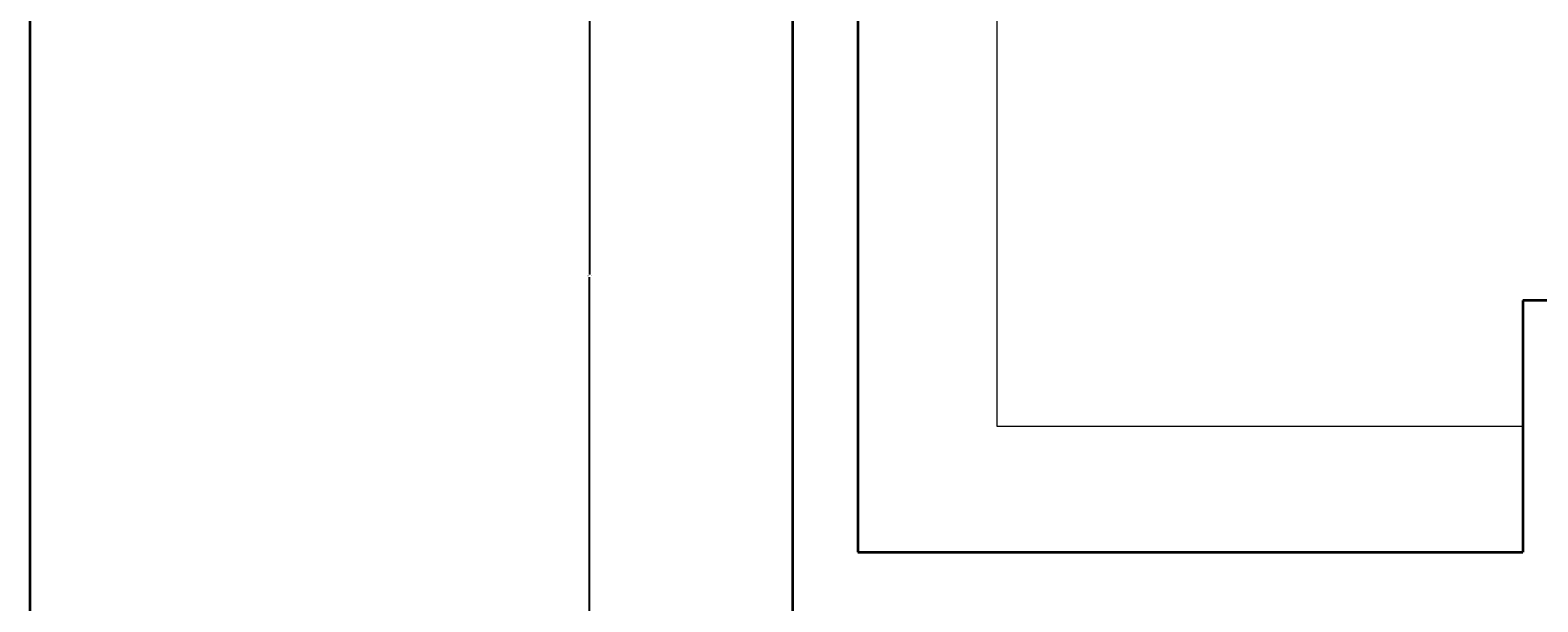
# Model space of a CAD drawing. Units: inches. Extents: x 1911 to 3278, y 2022 to 3108.
# Tile 6 of 13: x 1911 to 2120, y 2266 to 2345. Entities that reach past the tile are written whole.
import ezdxf

# ---------------------------------------------------------------- set-up
doc = ezdxf.new("R2010")
doc.units = ezdxf.units.IN
for name, color, linetype, lineweight in [('A-ANNO-DIMS', 2, 'Continuous', 18), ('A-ANNO-TTLB', 7, 'Continuous', 35), ('A-FLOR-CASE', 9, 'Continuous', 18), ('A-WALL', 7, 'Continuous', 35)]:
    doc.layers.add(name, color=color, linetype=linetype, lineweight=lineweight)
doc.styles.get("Standard").update_dxf_attribs({"font": 'arial.ttf'})
doc.dimstyles.get("Standard").update_dxf_attribs({"dimtxt": 0.18, "dimasz": 0.18, "dimexe": 0.18, "dimexo": 0.0625, "dimgap": 0.09, "dimtad": 0, "dimtih": 1, "dimtoh": 1, "dimdec": 4, "dimzin": 0, "dimdsep": 46, "dimtxsty": 'Standard', "dimcen": 0.09, "dimadec": 0, "dimazin": 0, "dimtfac": 1, "dimtdec": 4, "dimtofl": 0, "dimtmove": 0, "dimatfit": 3, "dimfxl": 1, "dimtolj": 1, "dimtzin": 0, "dimarcsym": 0})

# ---------------------------------------------------------------- blocks, each defined once
blk = doc.blocks.new('COUNTER-KITCHEN-L')
for p, q in [((19.27, 79.32), (0, 79.32)), ((19.27, 0), (19.27, 79.32)), ((92, 0), (19.27, 0))]:
    blk.add_line(p, q)
blk = doc.blocks.new('*D72')
at = {"layer": 'A-ANNO-DIMS', "color": 0, "lineweight": -2, "transparency": 16777216}
for p, q in [((2016.77, 2358.3), (1988.55, 2358.3)), ((1988.73, 2358.12), (1988.73, 2311.27)), ((1988.73, 2264.05), (1988.73, 2310.9)), ((2016.77, 2263.87), (1988.55, 2263.87))]:
    blk.add_line(p, q, dxfattribs=at)
at = {"layer": 'A-ANNO-DIMS', "color": 0, "transparency": 16777216}
for points in [[(1988.7, 2358.12), (1988.76, 2358.12), (1988.73, 2358.3)], [(1988.7, 2264.05), (1988.76, 2264.05), (1988.73, 2263.87)]]:
    blk.add_solid(points, dxfattribs=at)
at = {"layer": 'Defpoints', "color": 0, "transparency": 16777216}
for p in [(1988.73, 2358.3), (2016.83, 2358.3), (2016.83, 2263.87)]:
    blk.add_point(p, dxfattribs=at)
at = {"layer": 'A-ANNO-DIMS', "color": 0, "transparency": 16777216, "insert": (1988.73, 2311.09), "char_height": 0.18, "attachment_point": 5}
blk.add_mtext('\\A1;94.43', dxfattribs=at)

msp = doc.modelspace()

# ---------------------------------------------------------------- linework, layer by layer
at = {"layer": 'A-ANNO-TTLB'}
msp.add_lwpolyline([(1911.3875, 3108.0628), (3278.3142, 3108.0628), (3278.3142, 2021.7237), (1911.3875, 2021.7237)], close=True, dxfattribs=at)
at = {"layer": 'A-WALL'}
for p, q in [((2016.8344, 2620.8733), (2016.8344, 2133.8733)), ((2016.8344, 2620.8733), (2016.8344, 2133.8733)), ((2025.8344, 2549.3733), (2025.8344, 2272.8733)), ((2126.8344, 2307.6624), (2117.8344, 2307.6624)), ((2117.8344, 2307.6624), (2117.8344, 2272.8733)), ((2025.8344, 2272.8733), (2117.8344, 2272.8733))]:
    msp.add_line(p, q, dxfattribs=at)

# ---------------------------------------------------------------- block references
at = {"layer": 'A-FLOR-CASE'}
msp.add_blockref('COUNTER-KITCHEN-L', (2025.834, 2290.268), dxfattribs=at)

# ---------------------------------------------------------------- dimensions: what is measured, and where the dimension line sits
at = {"layer": 'A-ANNO-DIMS'}
dim = msp.add_linear_dim(base=(1988.7344, 2358.3003), p1=(2016.8344, 2263.8733), p2=(2016.8344, 2358.3003), angle=90, dimstyle='Standard', override={"dimdec": 2, "dimlfac": 1, "dimrnd": 0, "dimzin": 0, "dimdsep": 46, "dimlunit": 2}, dxfattribs=at)
dim.commit()
dim.dimension.update_dxf_attribs({"geometry": '*D72', "text_midpoint": (1988.7344, 2311.0868)})

doc.saveas('drawing.dxf')
